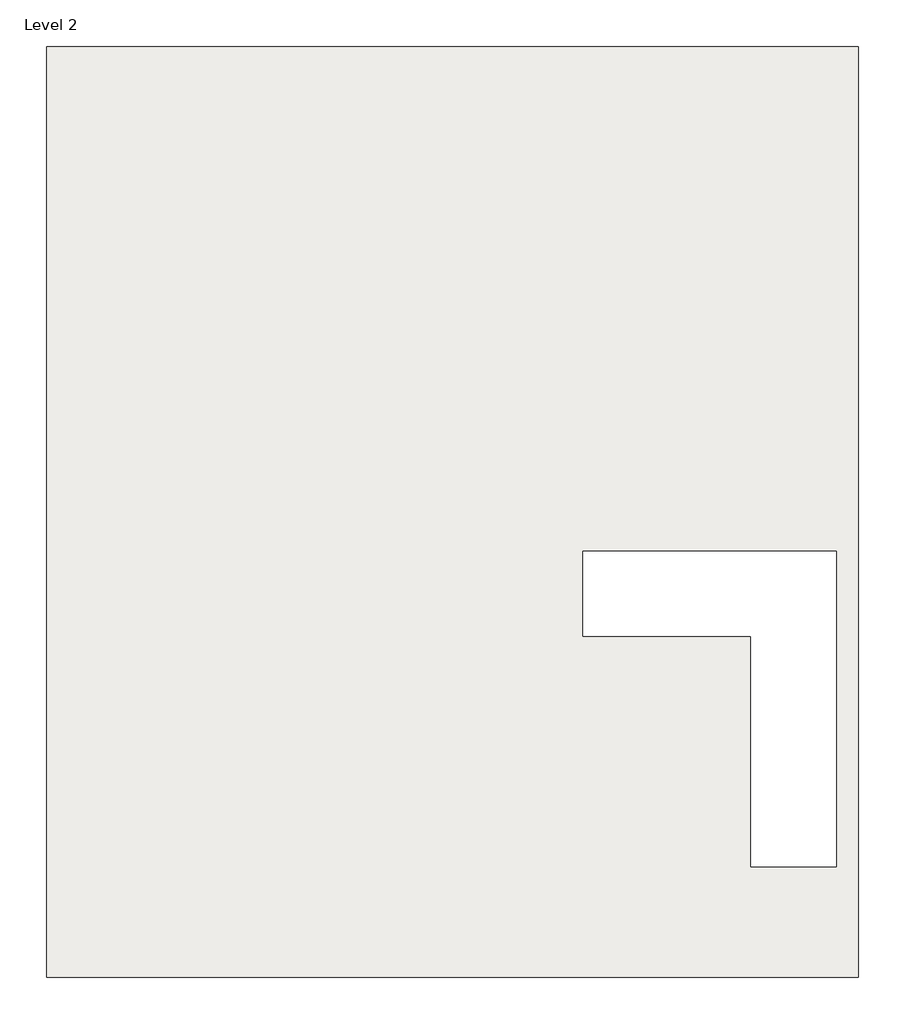
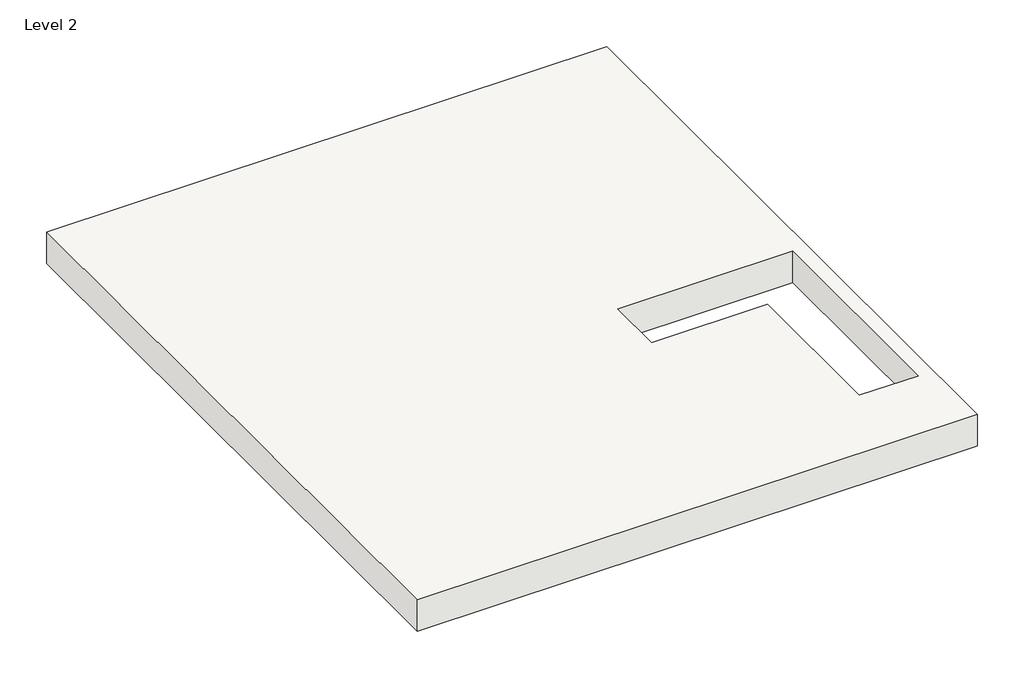
# One storey: 1 roof.
"""IFC4 building model written with IfcOpenShell, lengths in millimetres."""

from ifc_helpers import new_model, si_unit, frame, origin, place, context, project, spatial, polyline, outline, extrude, element, save

model = new_model("IFC4")

# Units and contexts
model_context = context("Model", 3, world=origin())
ifc_project = project(units=[si_unit("LENGTHUNIT", "METRE", prefix="MILLI")], contexts=[model_context])

# Site, building, storey
site = spatial("IfcSite", under=ifc_project)
building = spatial("IfcBuilding", under=site)
storey = spatial("IfcBuildingStorey", under=building, Name="Level 2", Elevation=3048.0)

# Roof
placement = place(None, origin())
element("IfcRoof", 1, ObjectType="Steel Truss - Insulation on Metal Deck - EPDM", at=placement, inside=storey, context=model_context, shape_type="SweptSolid", body=[
    extrude(outline(polyline([(-10148.5730118, 12638.9200123), (-953.7730118, 12638.9200123), (-953.7730118, 2097.9200123), (-10148.5730118, 2097.9200123), (-10148.5730118, 12638.9200123)]), holes=[polyline([(-4071.1932736, 6923.9200123), (-4071.1932736, 5958.7200123), (-2166.1932736, 5958.7200123), (-2166.1932736, 3353.09939), (-1200.9932736, 3353.09939), (-1200.9932736, 6923.9200123), (-4071.1932736, 6923.9200123)])]), frame((0.0, 0.0, 3048.0), z_axis=(0.0, 0.0, 1.0), x_axis=(1.0, 0.0, 0.0)), (0.0, 0.0, 1.0), 546.1),
])

save(model, "model.ifc")

# Revit data of these elements
# Type "Steel Truss - Insulation on Metal Deck - EPDM"
#   Assembly Code = "B1020"
#   Layers, outside or top first: 0' - 0 1/4" "Roofing, EPDM Membrane" (function 4); 0' - 5" "Rigid insulation" (function 3); 0' - 0 1/4" "Metal Deck" (function 1); 1' - 4" "Structure, Steel Bar Joist Layer" (function 1)
# Element 1 (IfcRoof, "Steel Truss - Insulation on Metal Deck - EPDM")
#   built-in parameter 1001705 = 11.7917 (stored number, unit not read)
#   built-in parameter 1001710 = 33615
#   Phase Created = New Construction
#   Materials on its faces: "Structure, Steel Bar Joist Layer", "Roofing, EPDM Membrane"
# Materials
#   "Roofing, EPDM Membrane": class "Generic", colour RGB 127 127 127, transparency 0, Description = "EPDM roof membrane", Cost = 0
#   "Rigid insulation": class "Generic", colour RGB 127 127 127, transparency 0, Description = "Rigid foam insulation board", Cost = 0
#   "Metal Deck": class "Metal", colour RGB 199 199 199, transparency 0, Description = "Steel, mill finish", Cost = 0
#   "Structure, Steel Bar Joist Layer": class "Metal", colour RGB 127 127 127, transparency 0, Description = "Bar joists, thermal airspace", Cost = 0
